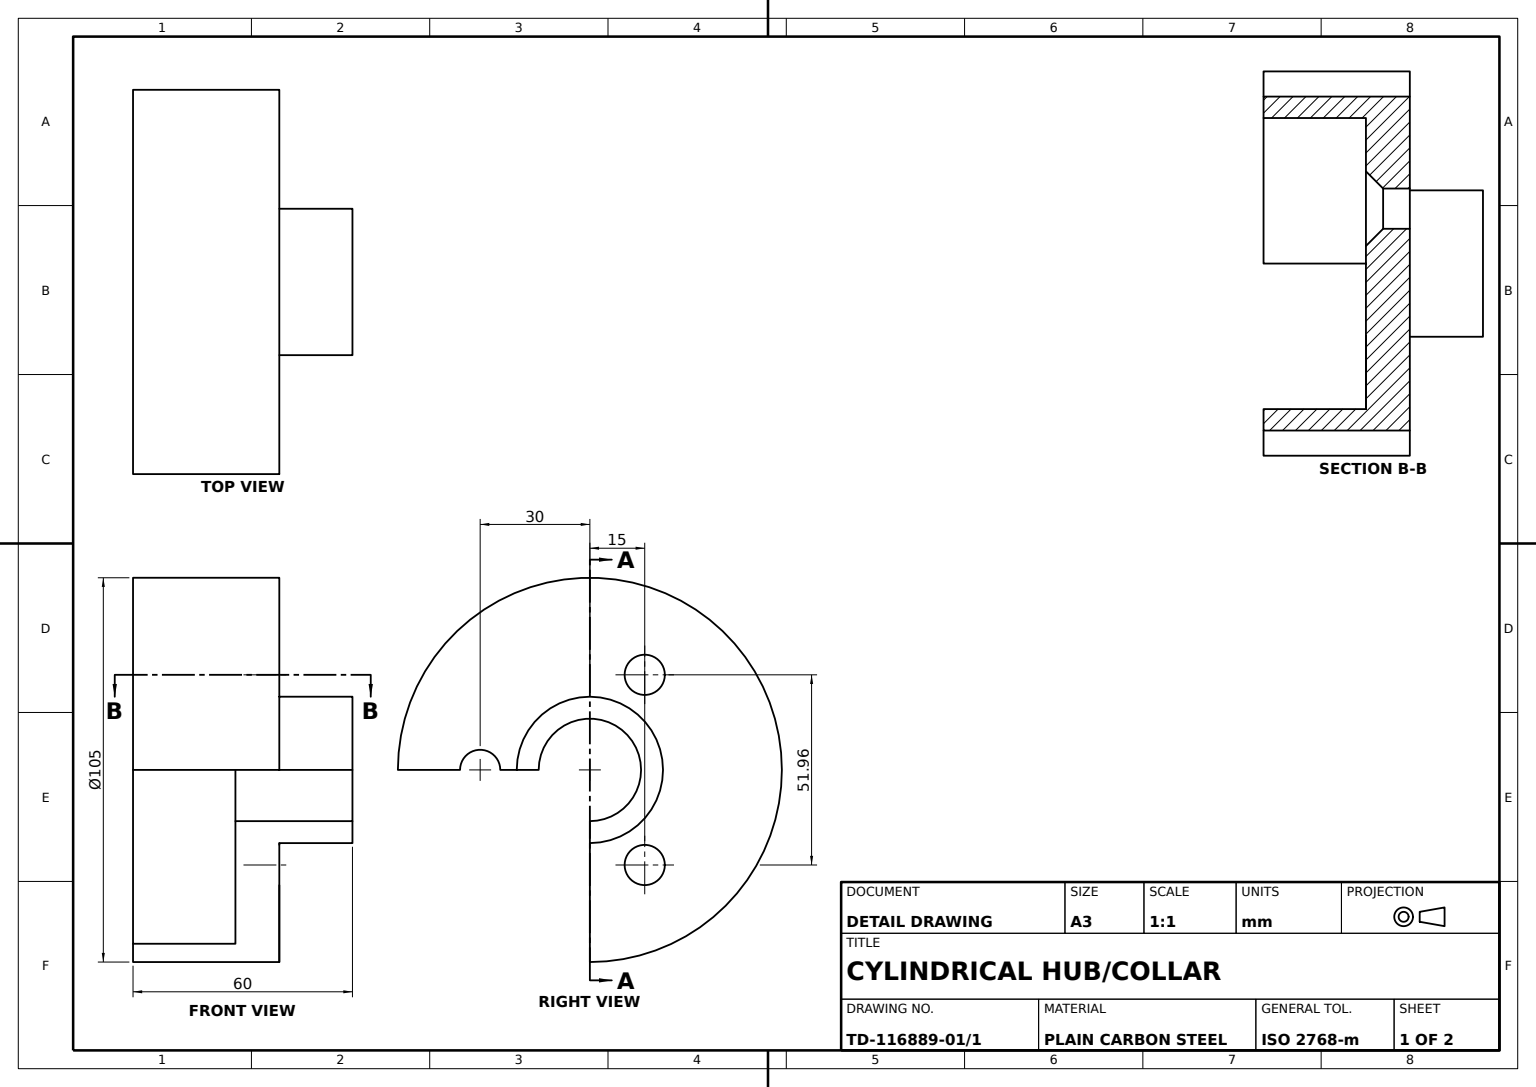
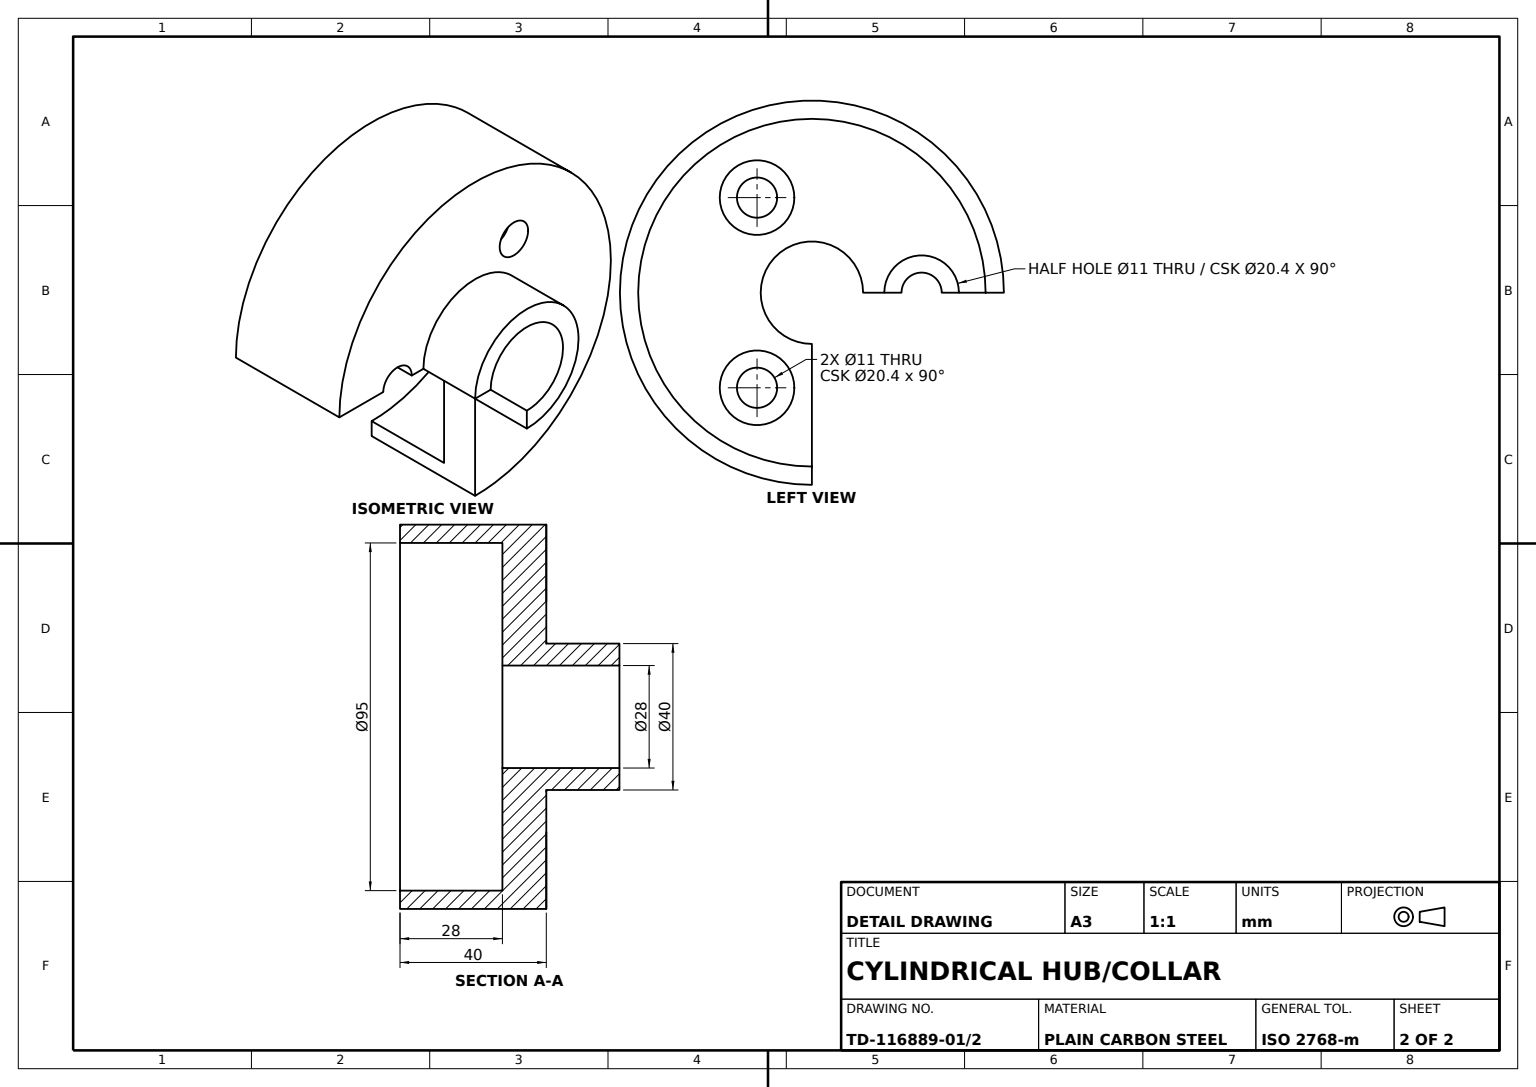
SolidWorks part; units mm, degrees
material "Plain Carbon Steel"
ref_plane "Front Plane" through (0, 0, 0) normal (0, 0, 1) x (1, 0, 0)
ref_plane "Top Plane" through (0, 0, 0) normal (0, 1, 0) x (1, 0, 0)
ref_plane "Right Plane" through (0, 0, 0) normal (1, 0, 0) x (0, 0, -1)
sketch "Bed Profile Sketch" plane through (0, 0, 0) normal (1, 0, 0) x (0, 0, -1)
  line L0 (0, 0) -> (0, 38.7613) construction
  line L1 (14, 30.3937) -> (14, -1.6063)
  line L2 (14, -1.6063) -> (47.5, -1.6063)
  line L3 (47.5, -1.6063) -> (47.5, -29.6063)
  line L4 (47.5, -29.6063) -> (52.5, -29.6063)
  line L5 (52.5, -29.6063) -> (52.5, 10.3937)
  line L6 (52.5, 10.3937) -> (20, 10.3937)
  line L7 (20, 10.3937) -> (20, 30.3937)
  line L8 (20, 30.3937) -> (14, 30.3937)
  dimension "D1" = 28
  dimension "D2" = 12
  dimension "D3" = 40
  dimension "D4" = 60
  dimension "D5" = 105
  dimension "D6" = 95
  dimension "D7" = 40
  dimension "D8" = 29.6063
revolve "Bed Body Revolve" add sketch "Bed Profile Sketch" angle 360 about L0
sketch "Hole Pitch Circle Ø60" plane through (0, -1.6063, 0) normal (0, -1, 0) x (1, 0, 0)
  circle A0 centre (0, 0) radius 30 construction
  point P3 (0, 30)
  dimension "D1" = 60
hole_wizard "Countersunk Hole Ø11" positions "3DSketch2" profile "Sketch4" countersink size "M4" standard "BSI" end condition through all
sketch3d "3DSketch2"
  point P0 (0, -1.6063, 30)
sketch "Sketch4" plane through (0, -1.6063, 30) normal (1, 0, 0) x (0, 0, -1)
  line L0 (0, 0) -> (0, 32)
  line L1 (0, 32) -> (5.5, 32)
  line L2 (5.5, 32) -> (5.5, 4.7)
  line L3 (5.5, 4.7) -> (10.2, 0)
  line L5 (10.2, 0) -> (0, 0)
  line L6 (-5.5, 4.7) -> (-10.2, 0) construction
  line L11 (0, -6.35) -> (0, 107.95) construction
  dimension "Thru Hole Dia." = 11
  dimension "Thru Hole Depth" = 32
  dimension "Near C'Sink Dia." = 20.4
  dimension "Near C'Sink Angle" = 90
pattern_circular "Countersunk Hole Pattern 3x" count 3 over 360 about axis through (0, 0, 0) along (0, 1, 0) of "Countersunk Hole Ø11"
sketch "Side Slot Sketch" plane through (0, -1.6063, 0) normal (0, -1, 0) x (1, 0, 0)
  line L0 (0, 66.3151) -> (0, 0)
  line L1 (0, 0) -> (70.3722, 0)
  arc A0 (0, 66.3151) -> (70.3722, 0) centre (11.8666, 8.4114) cw
  circle A1 centre (25.9808, -15) radius 10.2 construction
  dimension "D1" = 59.1071
  dimension "D2" = 44.3914
  dimension "D3" = 14.1141
extrude "Side Slot Cut" cut sketch "Side Slot Sketch" against normal through all both and the other way through all
